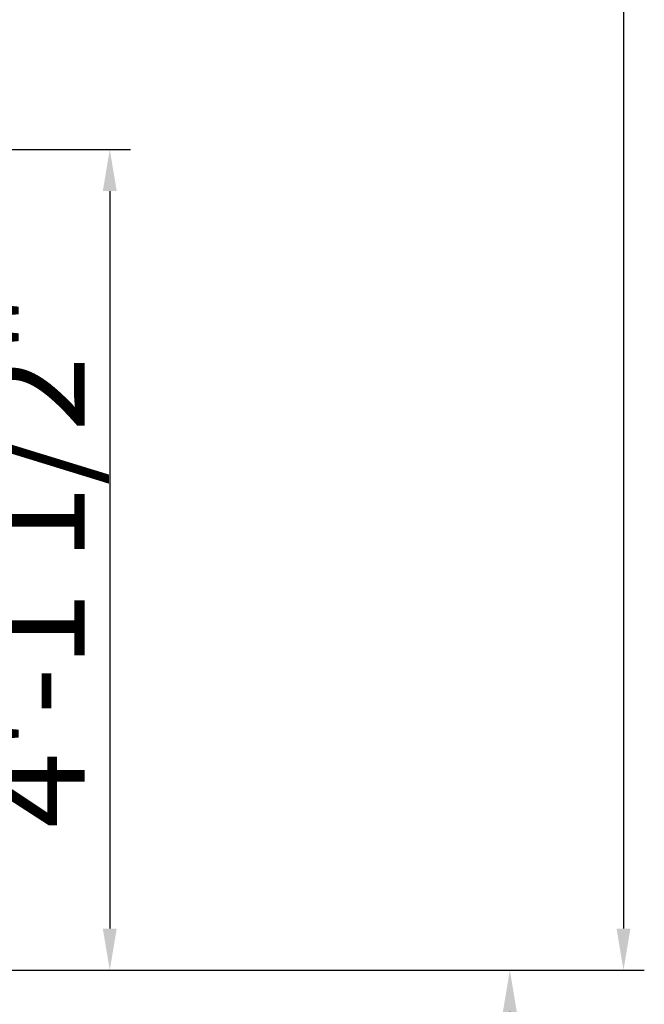
# Model space of a CAD drawing. Units: inches. Extents: x 459864 to 460310, y 324185 to 324787.
# Tile 108 of 112: x 460272 to 460310, y 324281 to 324341. Entities that reach past the tile are written whole.
import ezdxf

# ---------------------------------------------------------------- set-up
doc = ezdxf.new("R2010")
doc.units = ezdxf.units.IN
doc.layers.add('A-ANNO-DIMS', color=2, linetype='Continuous', lineweight=18)
doc.styles.get("Standard").update_dxf_attribs({"font": 'arial.ttf'})
doc.dimstyles.new('ISO-25', dxfattribs={"dimtxt": 6, "dimasz": 2.5, "dimexe": 1.25, "dimexo": 0.625, "dimtad": 1, "dimdec": 1, "dimlunit": 3, "dimtxsty": 'Standard', "dimcen": 2.5, "dimadec": 0, "dimazin": 0, "dimtfac": 1, "dimtdec": 1, "dimtmove": 0, "dimatfit": 3, "dimfxl": 1, "dimarcsym": 0})

# ---------------------------------------------------------------- blocks, each defined once
blk = doc.blocks.new('*D21')
at = {"layer": 'A-ANNO-DIMS', "color": 0, "lineweight": -2, "transparency": 16777216}
for p, q in [((460247.74, 324715.483), (460309.58, 324715.483)), ((460308.33, 324712.983), (460308.33, 324285.983)), ((460247.74, 324283.483), (460309.58, 324283.483))]:
    blk.add_line(p, q, dxfattribs=at)
at = {"layer": 'A-ANNO-DIMS', "color": 0, "transparency": 16777216}
for points in [[(460307.914, 324712.983), (460308.747, 324712.983), (460308.33, 324715.483)], [(460307.914, 324285.983), (460308.747, 324285.983), (460308.33, 324283.483)]]:
    blk.add_solid(points, dxfattribs=at)
at = {"layer": 'Defpoints', "color": 0, "transparency": 16777216}
for p in [(460247.115, 324715.483), (460247.115, 324283.483), (460308.33, 324283.483)]:
    blk.add_point(p, dxfattribs=at)
at = {"layer": 'A-ANNO-DIMS', "color": 0, "transparency": 16777216, "insert": (460304.64, 324499.483), "char_height": 6, "attachment_point": 5, "rotation": 90}
blk.add_mtext("36'", dxfattribs=at)
blk = doc.blocks.new('*D62')
at = {"layer": 'A-ANNO-DIMS', "color": 0, "lineweight": -2, "transparency": 16777216}
for p, q in [((460247.74, 324332.739), (460278.765, 324332.739)), ((460277.515, 324330.239), (460277.515, 324285.983)), ((460247.74, 324283.483), (460278.765, 324283.483))]:
    blk.add_line(p, q, dxfattribs=at)
at = {"layer": 'A-ANNO-DIMS', "color": 0, "transparency": 16777216}
for points in [[(460277.098, 324330.239), (460277.932, 324330.239), (460277.515, 324332.739)], [(460277.098, 324285.983), (460277.932, 324285.983), (460277.515, 324283.483)]]:
    blk.add_solid(points, dxfattribs=at)
at = {"layer": 'Defpoints', "color": 0, "transparency": 16777216}
for p in [(460247.115, 324332.739), (460247.115, 324283.483), (460277.515, 324283.483)]:
    blk.add_point(p, dxfattribs=at)
at = {"layer": 'A-ANNO-DIMS', "color": 0, "transparency": 16777216, "insert": (460273.788, 324308.111), "char_height": 6, "attachment_point": 5, "rotation": 90}
blk.add_mtext('4\'-1 1/2"', dxfattribs=at)
blk = doc.blocks.new('*D65')
at = {"layer": 'A-ANNO-DIMS', "color": 0, "lineweight": -2, "transparency": 16777216}
for p, q in [((460247.74, 324283.483), (460302.765, 324283.483)), ((460301.515, 324280.983), (460301.515, 324197.483)), ((460271.74, 324194.983), (460302.765, 324194.983))]:
    blk.add_line(p, q, dxfattribs=at)
at = {"layer": 'A-ANNO-DIMS', "color": 0, "transparency": 16777216}
for points in [[(460301.098, 324280.983), (460301.932, 324280.983), (460301.515, 324283.483)], [(460301.098, 324197.483), (460301.932, 324197.483), (460301.515, 324194.983)]]:
    blk.add_solid(points, dxfattribs=at)
at = {"layer": 'Defpoints', "color": 0, "transparency": 16777216}
for p in [(460247.115, 324283.483), (460271.115, 324194.983), (460301.515, 324194.983)]:
    blk.add_point(p, dxfattribs=at)
at = {"layer": 'A-ANNO-DIMS', "color": 0, "transparency": 16777216, "insert": (460297.788, 324239.233), "char_height": 6, "attachment_point": 5, "rotation": 90}
blk.add_mtext('7\'-4 1/2"', dxfattribs=at)

msp = doc.modelspace()

# ---------------------------------------------------------------- dimensions: what is measured, and where the dimension line sits
at = {"layer": 'A-ANNO-DIMS'}
for base, p1, p2, angle, override, picture, middle in [((460308.33, 324283.483), (460247.115, 324715.483), (460247.115, 324283.483), 90, {"dimclrd": 0, "dimclre": 0, "dimclrt": 0}, '*D21', (460304.64, 324499.483)), ((460277.515, 324283.483), (460247.115, 324332.739), (460247.115, 324283.483), 270, {"dimdec": 1, "dimlfac": 1, "dimrnd": 0, "dimzin": 1, "dimdsep": 46, "dimlunit": 4, "dimfrac": 2}, '*D62', (460273.788, 324308.111)), ((460301.515, 324194.983), (460247.115, 324283.483), (460271.115, 324194.983), 90, {"dimdec": 1, "dimlfac": 1, "dimrnd": 0, "dimzin": 1, "dimdsep": 46, "dimlunit": 4, "dimfrac": 2}, '*D65', (460297.788, 324239.233))]:
    dim = msp.add_linear_dim(base=base, p1=p1, p2=p2, angle=angle, dimstyle='ISO-25', override=override, dxfattribs=at)
    dim.commit()
    dim.dimension.update_dxf_attribs({"geometry": picture, "text_midpoint": middle})

doc.saveas('drawing.dxf')
